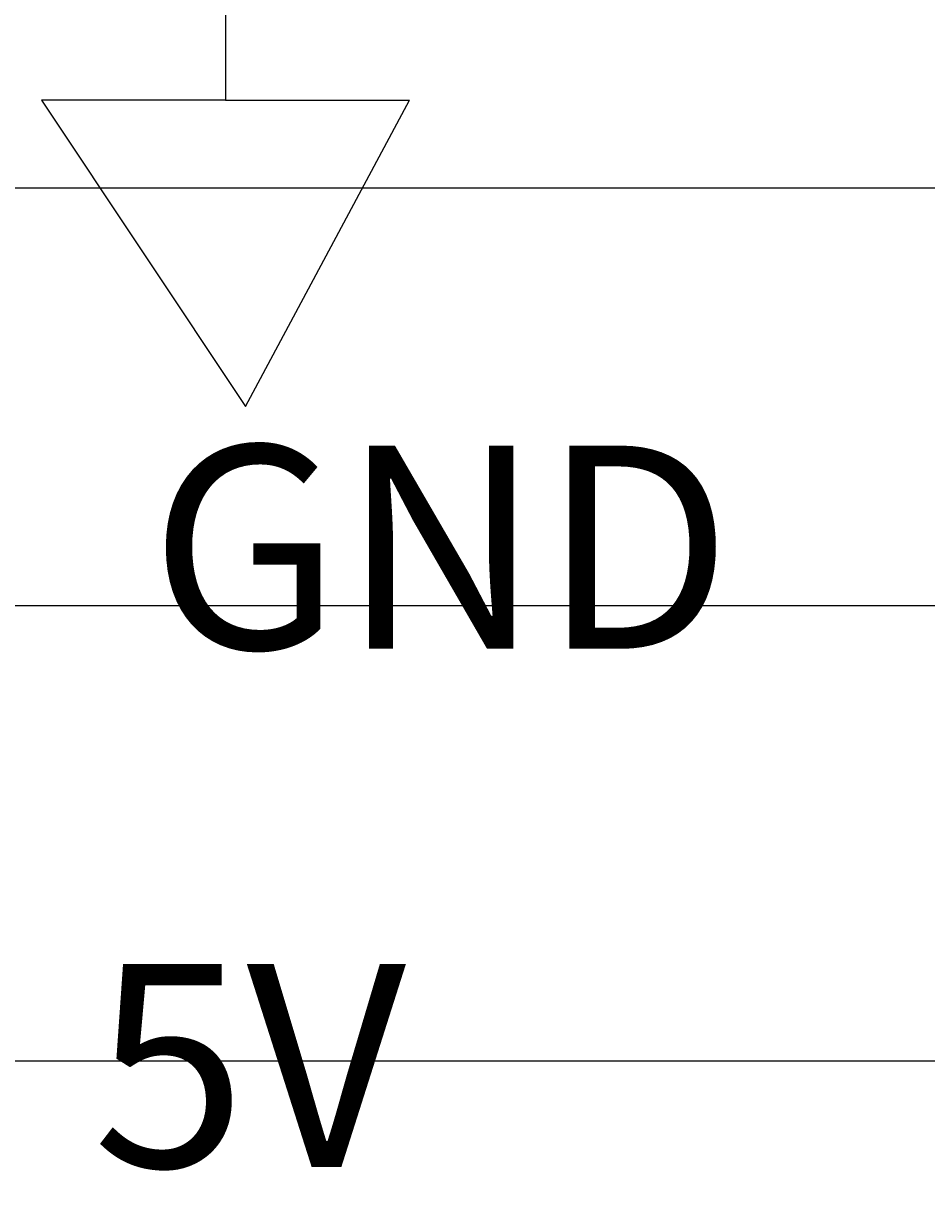
# Model space of a CAD drawing. Units: inches. Extents: x 35362 to 73946, y 43607 to 67532.
# Tile 134 of 134: x 68296 to 69277, y 55752 to 57027. Entities that reach past the tile are written whole.
import ezdxf

# ---------------------------------------------------------------- set-up
doc = ezdxf.new("R2010")
doc.units = ezdxf.units.IN
doc.header["$MEASUREMENT"] = 0
for name, color, linetype, lineweight in [('A-ANNO-DIMS', 2, 'Continuous', 18), ('E-ANNO-TEXT', 5, 'Continuous', 18), ('E-SYMB', 1, 'Continuous', 25)]:
    doc.layers.add(name, color=color, linetype=linetype, lineweight=lineweight)
doc.styles.get("Standard").update_dxf_attribs({"font": 'arial.ttf'})
doc.dimstyles.get("Standard").update_dxf_attribs({"dimtxt": 0.18, "dimasz": 0.18, "dimexe": 0.18, "dimexo": 0.0625, "dimgap": 0.09, "dimtad": 0, "dimtih": 1, "dimtoh": 1, "dimdec": 4, "dimzin": 0, "dimdsep": 46, "dimtxsty": 'Standard', "dimcen": 0.09, "dimadec": 0, "dimazin": 0, "dimtfac": 1, "dimtdec": 4, "dimtofl": 0, "dimtmove": 0, "dimatfit": 3, "dimfxl": 1, "dimtolj": 1, "dimtzin": 0, "dimarcsym": 0})

# ---------------------------------------------------------------- blocks, each defined once
blk = doc.blocks.new('*D8')
at = {"layer": 'A-ANNO-DIMS', "color": 0, "lineweight": -2, "transparency": 16777216}
for p, q in [((66271.28651900003, 65771.51172800003), (73945.82566600003, 65771.51172800003)), ((73945.64566600005, 65771.33172800003), (73945.64566600005, 59737.03093663782)), ((73945.64566600005, 53702.36633900002), (73945.64566600005, 59736.66713036224)), ((72185.70816600003, 53702.18633900003), (73945.82566600003, 53702.18633900003))]:
    blk.add_line(p, q, dxfattribs=at)
at = {"layer": 'A-ANNO-DIMS', "color": 0, "transparency": 16777216}
for points in [[(73945.61566600006, 65771.33172800003), (73945.67566600005, 65771.33172800003), (73945.64566600005, 65771.51172800003)], [(73945.61566600006, 53702.36633900002), (73945.67566600005, 53702.36633900002), (73945.64566600005, 53702.18633900003)]]:
    blk.add_solid(points, dxfattribs=at)
at = {"layer": 'Defpoints', "color": 0, "transparency": 16777216}
for p in [(66271.22401900003, 65771.51172800003), (73945.64566600005, 65771.51172800003), (72185.64566600003, 53702.18633900003)]:
    blk.add_point(p, dxfattribs=at)
at = {"layer": 'A-ANNO-DIMS', "color": 0, "transparency": 16777216, "insert": (73945.64566600005, 59736.84903349999), "char_height": 0.18, "attachment_point": 5}
blk.add_mtext('\\A1;12069', dxfattribs=at)
blk = doc.blocks.new('*D10')
at = {"layer": 'A-ANNO-DIMS', "color": 0, "lineweight": -2, "transparency": 16777216}
for p, q in [((61240.96983600002, 59185.14395700003), (73945.82566600003, 59185.14395700003)), ((73945.64566600005, 59184.96395700003), (73945.64566600005, 56268.51827402935)), ((73945.64566600005, 53351.70866200003), (73945.64566600005, 56268.1543449707)), ((61240.96983600002, 53351.52866200003), (73945.82566600003, 53351.52866200003))]:
    blk.add_line(p, q, dxfattribs=at)
at = {"layer": 'A-ANNO-DIMS', "color": 0, "transparency": 16777216}
for points in [[(73945.61566600006, 59184.96395700003), (73945.67566600005, 59184.96395700003), (73945.64566600005, 59185.14395700003)], [(73945.61566600006, 53351.70866200003), (73945.67566600005, 53351.70866200003), (73945.64566600005, 53351.52866200003)]]:
    blk.add_solid(points, dxfattribs=at)
at = {"layer": 'Defpoints', "color": 0, "transparency": 16777216}
for p in [(61240.90733600002, 59185.14395700003), (61240.90733600002, 53351.52866200003), (73945.64566600005, 53351.52866200003)]:
    blk.add_point(p, dxfattribs=at)
at = {"layer": 'A-ANNO-DIMS', "color": 0, "transparency": 16777216, "insert": (73945.64566600005, 56268.33630949999), "char_height": 0.18, "attachment_point": 5}
blk.add_mtext('\\A1;5834', dxfattribs=at)
blk = doc.blocks.new('*D36')
at = {"layer": 'A-ANNO-DIMS', "color": 0, "lineweight": -2, "transparency": 16777216}
for p, q in [((68320.80826200004, 60122.34633200002), (35361.76908500003, 60122.34633200002)), ((35361.94908500003, 60122.16633200002), (35361.94908500003, 57247.82893113781)), ((35361.94908500003, 54373.12772400002), (35361.94908500003, 57247.46512486223)), ((68320.80826200004, 54372.94772400003), (35361.76908500003, 54372.94772400002))]:
    blk.add_line(p, q, dxfattribs=at)
at = {"layer": 'A-ANNO-DIMS', "color": 0, "transparency": 16777216}
for points in [[(35361.91908500003, 60122.16633200002), (35361.97908500003, 60122.16633200002), (35361.94908500003, 60122.34633200002)], [(35361.91908500003, 54373.12772400002), (35361.97908500003, 54373.12772400002), (35361.94908500003, 54372.94772400002)]]:
    blk.add_solid(points, dxfattribs=at)
at = {"layer": 'Defpoints', "color": 0, "transparency": 16777216}
for p in [(68320.87076200004, 60122.34633200002), (35361.94908500003, 54372.94772400002), (68320.87076200004, 54372.94772400003)]:
    blk.add_point(p, dxfattribs=at)
at = {"layer": 'A-ANNO-DIMS', "color": 0, "transparency": 16777216, "insert": (35361.94908500004, 57247.64702799999), "char_height": 0.18, "attachment_point": 5}
blk.add_mtext('\\A1;5749.4', dxfattribs=at)
blk = doc.blocks.new('*D47')
at = {"layer": 'A-ANNO-DIMS', "color": 0, "lineweight": -2, "transparency": 16777216}
for p, q in [((50339.58680000003, 58279.98849500002), (73945.82566600003, 58279.98849500002)), ((73945.64566600005, 58279.80849500002), (73945.64566600005, 57564.17141502935)), ((73945.64566600005, 56848.17040600003), (73945.64566600005, 57563.80748597069)), ((50339.58680000003, 56847.99040600003), (73945.82566600003, 56847.99040600003))]:
    blk.add_line(p, q, dxfattribs=at)
at = {"layer": 'A-ANNO-DIMS', "color": 0, "transparency": 16777216}
for points in [[(73945.61566600006, 58279.80849500002), (73945.67566600005, 58279.80849500002), (73945.64566600005, 58279.98849500002)], [(73945.61566600006, 56848.17040600003), (73945.67566600005, 56848.17040600003), (73945.64566600005, 56847.99040600003)]]:
    blk.add_solid(points, dxfattribs=at)
at = {"layer": 'Defpoints', "color": 0, "transparency": 16777216}
for p in [(50339.52430000002, 58279.98849500002), (50339.52430000002, 56847.99040600003), (73945.64566600005, 56847.99040600003)]:
    blk.add_point(p, dxfattribs=at)
at = {"layer": 'A-ANNO-DIMS', "color": 0, "transparency": 16777216, "insert": (73945.64566600005, 57563.98945049999), "char_height": 0.18, "attachment_point": 5}
blk.add_mtext('\\A1;1432.0', dxfattribs=at)
blk = doc.blocks.new('*D50')
at = {"layer": 'A-ANNO-DIMS', "color": 0, "lineweight": -2, "transparency": 16777216}
for p, q in [((61657.28213900003, 56394.41825000003), (73945.82566600003, 56394.41825000003)), ((73945.64566600005, 56394.23825000003), (73945.64566600005, 56147.19337413782)), ((73945.64566600005, 55899.78469200003), (73945.64566600005, 56146.82956786224)), ((61657.28213900003, 55899.60469200002), (73945.82566600003, 55899.60469200002))]:
    blk.add_line(p, q, dxfattribs=at)
at = {"layer": 'A-ANNO-DIMS', "color": 0, "transparency": 16777216}
for points in [[(73945.61566600006, 56394.23825000003), (73945.67566600005, 56394.23825000003), (73945.64566600005, 56394.41825000003)], [(73945.61566600006, 55899.78469200003), (73945.67566600005, 55899.78469200003), (73945.64566600005, 55899.60469200002)]]:
    blk.add_solid(points, dxfattribs=at)
at = {"layer": 'Defpoints', "color": 0, "transparency": 16777216}
for p in [(61657.21963900003, 56394.41825000003), (61657.21963900003, 55899.60469200002), (73945.64566600005, 55899.60469200002)]:
    blk.add_point(p, dxfattribs=at)
at = {"layer": 'A-ANNO-DIMS', "color": 0, "transparency": 16777216, "insert": (73945.64566600005, 56147.01147099999), "char_height": 0.18, "attachment_point": 5}
blk.add_mtext('\\A1;494.8', dxfattribs=at)

msp = doc.modelspace()

# ---------------------------------------------------------------- linework, layer by layer
at = {"layer": 'E-SYMB'}
for p, q in [((68515.4609857722, 57372.14289754818), (68515.4609857722, 56943.54211886489)), ((68515.4609857722, 56943.54211886489), (68315.4609857722, 56943.54211886489)), ((68315.4609857722, 56943.54211886489), (68537.17167350776, 56610.60913620349)), ((68515.4609857722, 56943.54211886489), (68715.4609857722, 56943.54211886489)), ((68537.17167350776, 56610.60913620349), (68715.4609857722, 56943.54211886489))]:
    msp.add_line(p, q, dxfattribs=at)

# ---------------------------------------------------------------- texts
at = {"layer": 'E-ANNO-TEXT'}
for s, p in [('GND', (68433.1589458499, 56347.18317199525)), ('5V', (68371.01308383144, 55783.97972371984))]:
    msp.add_text(s, height=220.8659825270206, dxfattribs=at).set_placement(p)

# ---------------------------------------------------------------- dimensions: what is measured, and where the dimension line sits
at = {"layer": 'A-ANNO-DIMS'}
for base, p1, p2, override, picture, middle in [((73945.64566600005, 65771.51172800003), (72185.645666, 53702.186339), (66271.224019, 65771.51172799998), {"dimdec": 0, "dimlfac": 1, "dimrnd": 0, "dimzin": 0, "dimdsep": 46, "dimlunit": 2}, '*D8', (73945.64566600005, 59736.84903349999)), ((35361.94908500003, 54372.94772400002), (68320.870762, 60122.346332), (68320.870762, 54372.947724), {"dimdec": 1, "dimlfac": 1, "dimrnd": 0, "dimzin": 0, "dimdsep": 46, "dimlunit": 2}, '*D36', (35361.94908500004, 57247.64702799999)), ((73945.64566600005, 53351.52866200003), (61240.907336, 59185.14395699999), (61240.907336, 53351.52866199999), {"dimdec": 0, "dimlfac": 1, "dimrnd": 0, "dimzin": 0, "dimdsep": 46, "dimlunit": 2}, '*D10', (73945.64566600005, 56268.33630949999)), ((73945.64566600005, 56847.99040600003), (50339.5243, 58279.988495), (50339.5243, 56847.99040599999), {"dimdec": 1, "dimlfac": 1, "dimrnd": 0, "dimzin": 0, "dimdsep": 46, "dimlunit": 2}, '*D47', (73945.64566600005, 57563.98945049999)), ((73945.64566600005, 55899.60469200002), (61657.219639, 56394.41825), (61657.219639, 55899.604692), {"dimdec": 1, "dimlfac": 1, "dimrnd": 0, "dimzin": 0, "dimdsep": 46, "dimlunit": 2}, '*D50', (73945.64566600005, 56147.01147099999))]:
    dim = msp.add_linear_dim(base=base, p1=p1, p2=p2, angle=90, dimstyle='Standard', override=override, dxfattribs=at)
    dim.commit()
    dim.dimension.update_dxf_attribs({"geometry": picture, "text_midpoint": middle})

doc.saveas('drawing.dxf')
